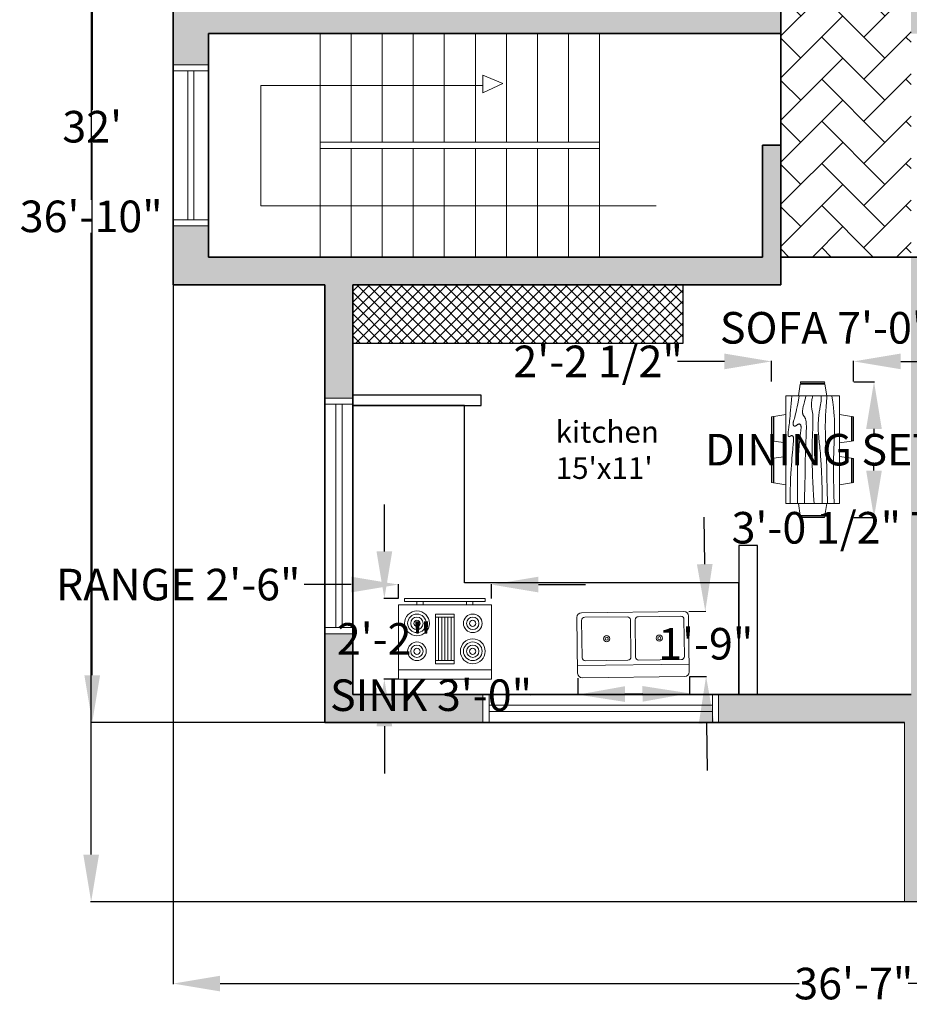
# Model space of a CAD drawing. Units: inches. Extents: x 1031 to 1706, y 87 to 654.
# Tile 1 of 4: x 1031 to 1318, y 96 to 413. Entities that reach past the tile are written whole.
import ezdxf

# ---------------------------------------------------------------- set-up
doc = ezdxf.new("R2010")
doc.units = ezdxf.units.IN
doc.header["$MEASUREMENT"] = 0
for name, color, linetype, lineweight in [('A-ANNO-DIMS', 2, 'Continuous', 18), ('A-ANNO-SYMB', 7, 'Continuous', 18), ('A-AREA-IDEN', 7, 'Continuous', 25), ('A-EQPM', 9, 'Continuous', 18), ('A-FLOR-CASE', 8, 'Continuous', 25), ('A-FLOR-CASE-PATT', 152, 'Continuous', 13), ('A-FLOR-FIXT', 114, 'Continuous', 18), ('A-FLOR-PATT', 152, 'Continuous', 13), ('A-FLOR-STRS', 7, 'Continuous', 18), ('A-FURN', 215, 'Continuous', 18), ('A-GLAZ', 4, 'Continuous', 18), ('A-WALL', 7, 'Continuous', 35), ('A-WALL-PATT', 18, 'Continuous', 13)]:
    doc.layers.add(name, color=color, linetype=linetype, lineweight=lineweight)
doc.styles.get("Standard").update_dxf_attribs({"font": 'arial.ttf'})
doc.dimstyles.get("Standard").update_dxf_attribs({"dimtxt": 10.18, "dimasz": 15.18, "dimexe": 0.18, "dimexo": 0.0625, "dimgap": 0.09, "dimtad": 0, "dimtih": 1, "dimtoh": 1, "dimdec": 0, "dimzin": 0, "dimdsep": 46, "dimlunit": 3, "dimtxsty": 'Standard', "dimcen": 0.09, "dimadec": 0, "dimazin": 0, "dimtfac": 1, "dimtdec": 0, "dimtofl": 0, "dimtmove": 0, "dimatfit": 3, "dimfxl": 1, "dimtolj": 1, "dimtzin": 0, "dimarcsym": 0})

# ---------------------------------------------------------------- blocks, each defined once
blk = doc.blocks.new('Dining Set - 36 x 72 in.')
for p, q in [((-22, 27.5), (-22.1562, 26.50042)), ((-5.8416, 26.5), (-22.1534, 26.5)), ((-22, 27.5), (-6, 27.5)), ((-5.8437, 26.49966), (-6, 27.5)), ((6, 27.5), (5.8438, 26.50042)), ((22.1584, 26.5), (5.8466, 26.5)), ((6, 27.5), (22, 27.5)), ((22.1563, 26.49966), (22, 27.5)), ((-22.2343, 26.00059), (-23.4847, 17.99762)), ((-22.2304, 26), (-5.7608, 26)), ((-4.5152, 17.99762), (-5.7655, 25.99926)), ((5.7657, 26.00059), (4.5153, 17.99762)), ((5.7696, 26), (22.2392, 26)), ((23.4848, 17.99762), (22.2345, 25.99926)), ((36, 18), (-36, 18)), ((-36, 18), (-36, -18)), ((36, -18), (36, 18)), ((-45.5, 8), (-44.5004, 8.15617)), ((-45.5, 8), (-45.5, -8)), ((-44.5, -8.15843), (-44.5, 8.15338)), ((-44.0006, 8.23428), (-35.9976, 9.48474)), ((-44, 8.23041), (-44, -8.23915)), ((44.0006, 8.23428), (35.9976, 9.48474)), ((44, 8.23041), (44, -8.23915)), ((44.5, -8.15843), (44.5, 8.15338)), ((45.5, 8), (44.5005, 8.15617)), ((45.5, 8), (45.5, -8)), ((-44.4997, -8.15631), (-45.5, -8)), ((-35.9976, -9.48476), (-43.9993, -8.2345)), ((35.9976, -9.48476), (43.9993, -8.2345)), ((44.4997, -8.15631), (45.5, -8)), ((-36, -18), (36, -18)), ((-22.2343, -26.0006), (-23.4847, -17.99762)), ((-4.5152, -17.99762), (-5.7655, -25.99928)), ((5.7657, -26.0006), (4.5153, -17.99762)), ((23.4848, -17.99762), (22.2345, -25.99928)), ((-22.2304, -26), (-5.7608, -26)), ((5.7696, -26), (22.2392, -26)), ((-22, -27.5), (-22.1562, -26.50044)), ((-5.8416, -26.5), (-22.1534, -26.5)), ((-22, -27.5), (-6, -27.5)), ((-5.8437, -26.49967), (-6, -27.5)), ((6, -27.5), (5.8438, -26.50044)), ((22.1584, -26.5), (5.8466, -26.5)), ((6, -27.5), (22, -27.5)), ((22.1563, -26.49967), (22, -27.5))]:
    blk.add_line(p, q)
for points in [[(-36, 15), (-31.1772, 14.97754), (-26.8079, 14.91406), (-22.8538, 14.81543), (-19.276, 14.6875), (-16.0362, 14.53613), (-13.0957, 14.36718), (-10.4159, 14.18652), (-7.9583, 14), (-5.6904, 13.81315), (-3.6035, 13.63021), (-1.6954, 13.45508), (0.0365, 13.29166), (1.5945, 13.14388), (2.9811, 13.01562), (4.1988, 12.9108), (5.25, 12.83333), (6.1393, 12.78613), (6.8802, 12.76823), (7.4883, 12.77767), (7.9792, 12.8125), (8.3685, 12.87077), (8.6719, 12.95052), (8.9049, 13.0498), (9.0833, 13.16666), (9.2205, 13.29899), (9.3216, 13.44401), (9.3895, 13.59879), (9.4271, 13.76041), (9.4373, 13.92594), (9.4232, 14.09245), (9.3875, 14.257), (9.3333, 14.41666), (9.2638, 14.56917), (9.1836, 14.71484), (9.0975, 14.85465), (9.0104, 14.98958), (8.9272, 15.1206), (8.8529, 15.2487), (8.7922, 15.37483), (8.75, 15.5), (8.7305, 15.62467), (8.7344, 15.74739), (8.7617, 15.86621), (8.8125, 15.97916), (8.8867, 16.08431), (8.9844, 16.17968), (9.1055, 16.26334), (9.25, 16.33333), (9.4189, 16.38802), (9.6172, 16.42708), (9.8506, 16.45052), (10.125, 16.45833), (10.4463, 16.45052), (10.8203, 16.42708), (11.2529, 16.38802), (11.75, 16.33333), (12.3184, 16.26318), (12.9694, 16.17838), (13.7151, 16.07991), (14.5677, 15.96875), (15.5395, 15.84586), (16.6426, 15.71224), (17.8893, 15.56884), (19.2917, 15.41666), (20.859, 15.25667), (22.5879, 15.08984), (24.4721, 14.91715), (26.5052, 14.73958), (28.6809, 14.5581), (30.9929, 14.3737), (33.4347, 14.18733), (36, 14)], [(-36, 10), (-28.9766, 10.14274), (-23.1725, 10.20442), (-18.4241, 10.19775), (-14.5677, 10.13541), (-11.4399, 10.03011), (-8.877, 9.89453), (-6.7154, 9.74137), (-4.7917, 9.58333), (-2.9698, 9.43082), (-1.2246, 9.28515), (0.4415, 9.14534), (2.026, 9.01041), (3.5266, 8.87939), (4.9408, 8.7513), (6.266, 8.62516), (7.5, 8.5), (8.6411, 8.37549), (9.6914, 8.2539), (10.6538, 8.13818), (11.5312, 8.03125), (12.3267, 7.93603), (13.043, 7.85547), (13.6831, 7.79248), (14.25, 7.75), (14.7471, 7.7303), (15.1797, 7.73307), (15.5537, 7.75732), (15.875, 7.80208), (16.1494, 7.86637), (16.3828, 7.94922), (16.5811, 8.04964), (16.75, 8.16666), (16.8944, 8.29915), (17.0143, 8.44531), (17.1089, 8.60319), (17.1771, 8.77083), (17.218, 8.94629), (17.2305, 9.1276), (17.2137, 9.31282), (17.1667, 9.5), (17.0895, 9.6875), (16.987, 9.875), (16.8649, 10.0625), (16.7292, 10.25), (16.5856, 10.4375), (16.4401, 10.625), (16.2985, 10.8125), (16.1667, 11), (16.05, 11.18733), (15.9518, 11.3737), (15.8752, 11.5581), (15.8229, 11.73958), (15.798, 11.91715), (15.8034, 12.08984), (15.842, 12.25667), (15.9167, 12.41666), (16.0295, 12.56836), (16.1784, 12.70833), (16.3605, 12.83268), (16.5729, 12.9375), (16.8127, 13.01888), (17.0768, 13.07291), (17.3625, 13.0957), (17.6667, 13.08333), (17.9894, 13.03312), (18.3418, 12.94726), (18.7382, 12.82918), (19.1927, 12.68229), (19.7195, 12.51001), (20.3327, 12.31575), (21.0465, 12.10294), (21.875, 11.875), (22.8357, 11.63354), (23.959, 11.37304), (25.2786, 11.08618), (26.8282, 10.76562), (28.6414, 10.40405), (30.752, 9.99414), (33.1936, 9.52856), (36, 9)], [(-36, 5.5), (-30.7157, 5.3348), (-26.069, 5.20963), (-21.9946, 5.11767), (-18.4271, 5.05208), (-15.3009, 5.00602), (-12.5508, 4.97265), (-10.1112, 4.94515), (-7.9167, 4.91666), (-5.909, 4.88167), (-4.0586, 4.83984), (-2.3429, 4.79215), (-0.7396, 4.73958), (0.7739, 4.6831), (2.22, 4.6237), (3.6213, 4.56233), (5, 4.5), (6.373, 4.43782), (7.7344, 4.3776), (9.0723, 4.32129), (10.375, 4.27083), (11.6309, 4.22819), (12.8281, 4.19531), (13.9551, 4.17415), (15, 4.16666), (15.954, 4.17448), (16.819, 4.19791), (17.6001, 4.23698), (18.3021, 4.29166), (18.9299, 4.36198), (19.4883, 4.44791), (19.9823, 4.54948), (20.4167, 4.66666), (20.7969, 4.79899), (21.1302, 4.94401), (21.4245, 5.09879), (21.6875, 5.26041), (21.9271, 5.42594), (22.1511, 5.59245), (22.3672, 5.757), (22.5834, 5.91666), (22.8065, 6.06868), (23.0404, 6.21093), (23.2879, 6.34147), (23.5521, 6.45833), (23.8358, 6.55957), (24.142, 6.64323), (24.4735, 6.70735), (24.8334, 6.75), (25.2235, 6.76969), (25.642, 6.76692), (26.0858, 6.74267), (26.5521, 6.69791), (27.0379, 6.63362), (27.5404, 6.55078), (28.0565, 6.45036), (28.5834, 6.33333), (29.1242, 6.19987), (29.7071, 6.04687), (30.3661, 5.87044), (31.1354, 5.66666), (32.0493, 5.43164), (33.142, 5.16146), (34.4475, 4.85221), (36, 4.5)], [(-36, -1), (-30.7915, -0.6591), (-26.0195, -0.38216), (-21.6519, -0.16284), (-17.6563, 0.00521), (-14.0005, 0.12833), (-10.6523, 0.21289), (-7.5796, 0.26522), (-4.75, 0.29166), (-2.134, 0.29793), (0.2878, 0.28711), (2.5317, 0.26163), (4.6146, 0.22396), (6.5529, 0.17651), (8.3633, 0.12174), (10.0623, 0.06209), (11.6667, 0), (13.1899, -0.06201), (14.6341, -0.1211), (15.9982, -0.17432), (17.2813, -0.21875), (18.4823, -0.25147), (19.6003, -0.26953), (20.6343, -0.27002), (21.5834, -0.25), (22.4481, -0.20768), (23.2357, -0.14584), (23.9549, -0.06836), (24.6146, 0.02083), (25.2235, 0.11784), (25.7904, 0.21875), (26.3241, 0.31966), (26.8334, 0.41666), (27.3265, 0.50618), (27.8099, 0.58593), (28.2894, 0.65397), (28.7709, 0.70833), (29.2601, 0.74707), (29.763, 0.76823), (30.2855, 0.76985), (30.8334, 0.75), (31.4088, 0.70784), (31.9994, 0.64713), (32.589, 0.57275), (33.1615, 0.48958), (33.7008, 0.4025), (34.1908, 0.3164), (34.6153, 0.23616), (34.9584, 0.16666), (35.2099, 0.11165), (35.3848, 0.07031), (35.504, 0.04069), (35.5886, 0.02083), (35.6594, 0.00879), (35.7377, 0.0026), (35.8442, 0.00032), (36, 0)], [(-36, -6.5), (-27.1843, -6.31267), (-20.084, -6.1263), (-14.469, -5.9419), (-10.1094, -5.76042), (-6.7752, -5.58285), (-4.2363, -5.41016), (-2.2629, -5.24333), (-0.625, -5.08334), (0.8708, -4.93099), (2.2715, -4.78646), (3.5872, -4.64974), (4.8281, -4.52084), (6.0046, -4.39974), (7.127, -4.28646), (8.2053, -4.18099), (9.25, -4.08334), (10.2705, -3.99382), (11.2734, -3.91407), (12.2647, -3.84603), (13.25, -3.79167), (14.2354, -3.75293), (15.2266, -3.73177), (16.2295, -3.73015), (17.25, -3.75), (18.2912, -3.79248), (19.3451, -3.85547), (20.4009, -3.93604), (21.4479, -4.03125), (22.4754, -4.13819), (23.4727, -4.25391), (24.4289, -4.37549), (25.3334, -4.5), (26.1785, -4.62492), (26.9694, -4.74935), (27.7145, -4.87281), (28.4219, -4.99479), (29.1, -5.11483), (29.7572, -5.23242), (30.4016, -5.34709), (31.0417, -5.45834), (31.6837, -5.56437), (32.3262, -5.65821), (32.9658, -5.73153), (33.599, -5.77604), (34.2224, -5.78345), (34.8327, -5.74545), (35.4264, -5.65373), (36, -5.5)], [(-36, -10), (-26.4022, -9.81299), (-18.4675, -9.62891), (-11.9839, -9.45069), (-6.7396, -9.28125), (-2.5226, -9.12354), (0.8789, -8.98047), (3.6769, -8.85498), (6.0833, -8.75), (8.2767, -8.66765), (10.3021, -8.60677), (12.1712, -8.56543), (13.8958, -8.54167), (15.4876, -8.53353), (16.9583, -8.53907), (18.3197, -8.55632), (19.5834, -8.58334), (20.7616, -8.61841), (21.8685, -8.66081), (22.9188, -8.71004), (23.9271, -8.76563), (24.9081, -8.82707), (25.8763, -8.89388), (26.8465, -8.96558), (27.8334, -9.04167), (28.8474, -9.12118), (29.8828, -9.20117), (30.93, -9.27824), (31.9792, -9.34896), (33.0205, -9.40991), (34.0443, -9.45768), (35.0407, -9.48885), (36, -9.5)], [(-36, -14.5), (-30.0881, -14.33513), (-25.0332, -14.21224), (-20.7312, -14.12647), (-17.0781, -14.07292), (-13.97, -14.04671), (-11.3027, -14.04297), (-8.9724, -14.05681), (-6.875, -14.08334), (-4.9224, -14.11833), (-3.0905, -14.16016), (-1.3709, -14.20785), (0.2448, -14.26042), (1.7647, -14.3169), (3.1973, -14.3763), (4.5507, -14.43767), (5.8333, -14.5), (7.0554, -14.5621), (8.235, -14.62175), (9.3922, -14.67652), (10.5469, -14.72396), (11.7192, -14.76164), (12.929, -14.78711), (14.1965, -14.79794), (15.5417, -14.79167), (16.9933, -14.76424), (18.6152, -14.70508), (20.4804, -14.60197), (22.6615, -14.44271), (25.2312, -14.21509), (28.2624, -13.9069), (31.8277, -13.50594), (36, -13)]]:
    blk.add_lwpolyline(points)
blk = doc.blocks.new('Range-Oven - 30 in top')
for p, q in [((0, -3), (30, -3)), ((12, -6), (18, -6)), ((13, -20), (13, -6)), ((14, -6), (14, -20)), ((15, -20), (15, -6)), ((16, -6), (16, -20)), ((17, -20), (17, -6)), ((18, -20), (12, -20)), ((6, -24), (6, -25)), ((8, -25), (8, -24)), ((22, -25), (22, -24)), ((24, -24), (24, -25))]:
    blk.add_line(p, q)
for points in [[(0, -24), (0, 0), (30, 0), (30, -24)], [(12, -21), (12, -5), (18, -5), (18, -21)], [(2, -26), (2, -25), (28, -25), (28, -26)]]:
    blk.add_lwpolyline(points, close=True)
for centre, radius in [((6, -9), 4), ((6, -9), 3), ((24, -9), 3), ((6, -9), 2), ((6, -9), 1), ((24, -9), 2), ((24, -9), 1), ((6, -18), 3), ((24, -18), 4), ((24, -18), 3), ((6, -18), 2), ((6, -18), 1), ((24, -18), 2), ((24, -18), 1)]:
    blk.add_circle(centre, radius)
blk = doc.blocks.new('Sink-double - 36 in top')
for p, q in [((-18, -4), (18, -4)), ((-0.75, -18.5), (-0.75, -6.5)), ((0.75, -6.5), (0.75, -18.5))]:
    blk.add_line(p, q)
for points in [[(-16.5, 0), (16.5, 0)], [(-18, -19.5), (-18, -1.5)], [(18, -1.5), (18, -19.5)], [(-15.5, -5.5), (-1.75, -5.5)], [(1.75, -5.5), (15.5, -5.5)], [(-16.5, -18.5), (-16.5, -6.5)], [(16.5, -6.5), (16.5, -18.5)], [(16.5, -21), (-16.5, -21)], [(-1.75, -19.5), (-15.5, -19.5)], [(15.5, -19.5), (1.75, -19.5)]]:
    blk.add_lwpolyline(points)
for centre, radius in [((-8.5, -12.5), 1), ((-8.5, -12.5), 0.5), ((8.5, -12.5), 1), ((8.5, -12.5), 0.5)]:
    blk.add_circle(centre, radius)
for centre, radius, start, end in [((-16.5, -1.5), 1.5, 90, 180), ((16.5, -1.5), 1.5, 0, 90), ((-15.5, -6.5), 1, 90, 180), ((-1.75, -6.5), 1, 0, 90), ((1.75, -6.5), 1, 90, 180), ((15.5, -6.5), 1, 0, 90), ((-15.5, -18.5), 1, 180, 270), ((-1.75, -18.5), 1, 270, 0), ((1.75, -18.5), 1, 180, 270), ((15.5, -18.5), 1, 270, 0), ((-16.5, -19.5), 1.5, 180, 270), ((16.5, -19.5), 1.5, 270, 0)]:
    blk.add_arc(centre, radius, start, end)
blk = doc.blocks.new('*D13')
at = {"layer": 'A-ANNO-DIMS', "color": 0, "lineweight": -2, "transparency": 16777216}
for p, q in [((1129.54, 570.4), (1054.37, 570.4)), ((1054.55, 555.22), (1054.55, 383.69)), ((1054.55, 201.58), (1054.55, 373.11)), ((1129.54, 186.4), (1054.37, 186.4))]:
    blk.add_line(p, q, dxfattribs=at)
at = {"layer": 'A-ANNO-DIMS', "color": 0, "transparency": 16777216}
for points in [[(1052.02, 555.22), (1057.08, 555.22), (1054.55, 570.4)], [(1052.02, 201.58), (1057.08, 201.58), (1054.55, 186.4)]]:
    blk.add_solid(points, dxfattribs=at)
at = {"layer": 'Defpoints', "color": 0, "transparency": 16777216}
for p in [(1129.6, 570.4), (1054.55, 186.4), (1129.6, 186.4)]:
    blk.add_point(p, dxfattribs=at)
at = {"layer": 'A-ANNO-DIMS', "color": 0, "transparency": 16777216, "insert": (1054.55, 378.4), "char_height": 10.18, "attachment_point": 5}
blk.add_mtext("\\A1;32'", dxfattribs=at)
blk = doc.blocks.new('WIN-72IN')
for p, q in [((0, 0), (0, 9)), ((2, 0), (2, 9)), ((74, 0), (74, 9)), ((76, 0), (76, 9)), ((2, 5.5), (74, 5.5)), ((2, 3.5), (74, 3.5))]:
    blk.add_line(p, q)
blk = doc.blocks.new('*D28')
at = {"layer": 'A-ANNO-DIMS', "color": 0, "lineweight": -2, "transparency": 16777216}
for p, q in [((1374.5, 313.58), (1359.32, 313.58)), ((1374.5, 301.04), (1374.5, 313.76)), ((1443.32, 313.58), (1389.68, 313.58)), ((1458.5, 301.04), (1458.5, 313.76))]:
    blk.add_line(p, q, dxfattribs=at)
at = {"layer": 'A-ANNO-DIMS', "color": 0, "transparency": 16777216}
for points in [[(1389.68, 316.11), (1389.68, 311.05), (1374.5, 313.58)], [(1443.32, 316.11), (1443.32, 311.05), (1458.5, 313.58)]]:
    blk.add_solid(points, dxfattribs=at)
at = {"layer": 'Defpoints', "color": 0, "transparency": 16777216}
for p in [(1374.5, 313.58), (1374.5, 300.98), (1458.5, 300.98)]:
    blk.add_point(p, dxfattribs=at)
at = {"layer": 'A-ANNO-DIMS', "color": 0, "transparency": 16777216, "insert": (1306.9, 313.58), "char_height": 10.18, "attachment_point": 5}
blk.add_mtext('\\A1;SOFA 7\'-0" TYP.', dxfattribs=at)
blk = doc.blocks.new('*D29')
at = {"layer": 'A-ANNO-DIMS', "color": 0, "lineweight": -2, "transparency": 16777216}
for p, q in [((1374.44, 300.98), (1361.72, 300.98)), ((1361.9, 285.8), (1361.9, 279.49)), ((1374.44, 264.31), (1361.72, 264.31)), ((1361.9, 264.31), (1361.9, 249.13)), ((1361.9, 249.13), (1346.72, 249.13))]:
    blk.add_line(p, q, dxfattribs=at)
at = {"layer": 'A-ANNO-DIMS', "color": 0, "transparency": 16777216}
for points in [[(1359.37, 285.8), (1364.43, 285.8), (1361.9, 300.98)], [(1359.37, 279.49), (1364.43, 279.49), (1361.9, 264.31)]]:
    blk.add_solid(points, dxfattribs=at)
at = {"layer": 'Defpoints', "color": 0, "transparency": 16777216}
for p in [(1374.5, 300.98), (1361.9, 264.31), (1374.5, 264.31)]:
    blk.add_point(p, dxfattribs=at)
at = {"layer": 'A-ANNO-DIMS', "color": 0, "transparency": 16777216, "insert": (1303.75, 249.13), "char_height": 10.18, "attachment_point": 5}
blk.add_mtext('\\A1;3\'-0 1/2" TYP.', dxfattribs=at)
blk = doc.blocks.new('*D30')
at = {"layer": 'A-ANNO-DIMS', "color": 0, "lineweight": -2, "transparency": 16777216}
for p, q in [((1300.12, 296.19), (1306.8, 296.19)), ((1306.62, 281.01), (1306.62, 279.65)), ((1306.62, 267.58), (1306.62, 268.93)), ((1300.12, 252.4), (1306.8, 252.4))]:
    blk.add_line(p, q, dxfattribs=at)
at = {"layer": 'A-ANNO-DIMS', "color": 0, "transparency": 16777216}
for points in [[(1304.09, 281.01), (1309.15, 281.01), (1306.62, 296.19)], [(1304.09, 267.58), (1309.15, 267.58), (1306.62, 252.4)]]:
    blk.add_solid(points, dxfattribs=at)
at = {"layer": 'Defpoints', "color": 0, "transparency": 16777216}
for p in [(1300.06, 296.19), (1306.62, 296.19), (1300.06, 252.4)]:
    blk.add_point(p, dxfattribs=at)
at = {"layer": 'A-ANNO-DIMS', "color": 0, "transparency": 16777216, "insert": (1306.62, 274.29), "char_height": 10.18, "attachment_point": 5}
blk.add_mtext('\\A1;DINING SET 3\'-8"', dxfattribs=at)
blk = doc.blocks.new('*D31')
at = {"layer": 'A-ANNO-DIMS', "color": 0, "lineweight": -2, "transparency": 16777216}
for p, q in [((1258.41, 302.75), (1243.23, 302.75)), ((1273.59, 296.25), (1273.59, 302.93)), ((1300.06, 296.25), (1300.06, 302.93)), ((1315.24, 302.75), (1330.42, 302.75))]:
    blk.add_line(p, q, dxfattribs=at)
at = {"layer": 'A-ANNO-DIMS', "color": 0, "transparency": 16777216}
for points in [[(1258.41, 305.28), (1258.41, 300.22), (1273.59, 302.75)], [(1315.24, 305.28), (1315.24, 300.22), (1300.06, 302.75)]]:
    blk.add_solid(points, dxfattribs=at)
at = {"layer": 'Defpoints', "color": 0, "transparency": 16777216}
for p in [(1273.59, 302.75), (1273.59, 296.19), (1300.06, 296.19)]:
    blk.add_point(p, dxfattribs=at)
at = {"layer": 'A-ANNO-DIMS', "color": 0, "transparency": 16777216, "insert": (1217.66, 302.75), "char_height": 10.18, "attachment_point": 5}
blk.add_mtext('\\A1;2\'-2 1/2"', dxfattribs=at)
blk = doc.blocks.new('*D34')
at = {"layer": 'A-ANNO-DIMS', "color": 0, "lineweight": -2, "transparency": 16777216}
for p, q in [((1138.07, 230.82), (1122.89, 230.82)), ((1153.25, 226.38), (1153.25, 231)), ((1183.25, 226.38), (1183.25, 231)), ((1198.43, 230.82), (1213.61, 230.82))]:
    blk.add_line(p, q, dxfattribs=at)
at = {"layer": 'A-ANNO-DIMS', "color": 0, "transparency": 16777216}
for points in [[(1138.07, 233.35), (1138.07, 228.29), (1153.25, 230.82)], [(1198.43, 233.35), (1198.43, 228.29), (1183.25, 230.82)]]:
    blk.add_solid(points, dxfattribs=at)
at = {"layer": 'Defpoints', "color": 0, "transparency": 16777216}
for p in [(1153.25, 230.82), (1153.25, 226.32), (1183.25, 226.32)]:
    blk.add_point(p, dxfattribs=at)
at = {"layer": 'A-ANNO-DIMS', "color": 0, "transparency": 16777216, "insert": (1082.27, 230.82), "char_height": 10.18, "attachment_point": 5}
blk.add_mtext('\\A1;RANGE 2\'-6"', dxfattribs=at)
blk = doc.blocks.new('*D35')
at = {"layer": 'A-ANNO-DIMS', "color": 0, "lineweight": -2, "transparency": 16777216}
for p, q in [((1148.75, 241.5), (1148.75, 256.68)), ((1153.18, 226.32), (1148.57, 226.32)), ((1153.18, 200.32), (1148.57, 200.32)), ((1148.75, 185.14), (1148.75, 169.96))]:
    blk.add_line(p, q, dxfattribs=at)
at = {"layer": 'A-ANNO-DIMS', "color": 0, "transparency": 16777216}
for points in [[(1146.22, 241.5), (1151.28, 241.5), (1148.75, 226.32)], [(1146.22, 185.14), (1151.28, 185.14), (1148.75, 200.32)]]:
    blk.add_solid(points, dxfattribs=at)
at = {"layer": 'Defpoints', "color": 0, "transparency": 16777216}
for p in [(1153.25, 226.32), (1148.75, 200.32), (1153.25, 200.32)]:
    blk.add_point(p, dxfattribs=at)
at = {"layer": 'A-ANNO-DIMS', "color": 0, "transparency": 16777216, "insert": (1148.75, 213.32), "char_height": 10.18, "attachment_point": 5}
blk.add_mtext('\\A1;2\'-2"', dxfattribs=at)
blk = doc.blocks.new('*D36')
at = {"layer": 'A-ANNO-DIMS', "color": 0, "lineweight": -2, "transparency": 16777216}
for p, q in [((1211.08, 200.68), (1211.15, 195.16)), ((1247.08, 201.11), (1247.15, 195.59)), ((1211.15, 195.34), (1195.97, 195.16)), ((1231.97, 195.59), (1226.33, 195.52))]:
    blk.add_line(p, q, dxfattribs=at)
at = {"layer": 'A-ANNO-DIMS', "color": 0, "transparency": 16777216}
for points in [[(1226.3, 198.05), (1226.36, 192.99), (1211.15, 195.34)], [(1231.94, 198.12), (1232, 193.06), (1247.14, 195.77)]]:
    blk.add_solid(points, dxfattribs=at)
at = {"layer": 'Defpoints', "color": 0, "transparency": 16777216}
for p in [(1211.08, 200.74), (1247.08, 201.17), (1211.15, 195.34)]:
    blk.add_point(p, dxfattribs=at)
at = {"layer": 'A-ANNO-DIMS', "color": 0, "transparency": 16777216, "insert": (1163.8, 195.16), "char_height": 10.18, "attachment_point": 5}
blk.add_mtext('\\A1;SINK 3\'-0"', dxfattribs=at)
blk = doc.blocks.new('*D37')
at = {"layer": 'A-ANNO-DIMS', "color": 0, "lineweight": -2, "transparency": 16777216}
for p, q in [((1252.05, 237.41), (1251.87, 252.59)), ((1246.89, 222.17), (1252.41, 222.23)), ((1247.14, 201.17), (1252.66, 201.23)), ((1252.66, 186.05), (1252.84, 170.87))]:
    blk.add_line(p, q, dxfattribs=at)
at = {"layer": 'A-ANNO-DIMS', "color": 0, "transparency": 16777216}
for points in [[(1254.58, 237.44), (1249.52, 237.38), (1252.23, 222.23)], [(1255.19, 186.08), (1250.13, 186.02), (1252.48, 201.23)]]:
    blk.add_solid(points, dxfattribs=at)
at = {"layer": 'Defpoints', "color": 0, "transparency": 16777216}
for p in [(1246.83, 222.17), (1247.08, 201.17), (1252.48, 201.23)]:
    blk.add_point(p, dxfattribs=at)
at = {"layer": 'A-ANNO-DIMS', "color": 0, "transparency": 16777216, "insert": (1252.36, 211.73), "char_height": 10.18, "attachment_point": 5}
blk.add_mtext('\\A1;1\'-9"', dxfattribs=at)
blk = doc.blocks.new('*D40')
at = {"layer": 'A-ANNO-DIMS', "color": 0, "lineweight": -2, "transparency": 16777216}
for p, q in [((1080.61, 327.33), (1080.61, 102.02)), ((1519.6, 186.33), (1519.6, 102.02)), ((1095.79, 102.2), (1282.53, 102.2)), ((1504.42, 102.2), (1317.68, 102.2))]:
    blk.add_line(p, q, dxfattribs=at)
at = {"layer": 'A-ANNO-DIMS', "color": 0, "transparency": 16777216}
for points in [[(1095.79, 104.73), (1095.79, 99.67), (1080.61, 102.2)], [(1504.42, 104.73), (1504.42, 99.67), (1519.6, 102.2)]]:
    blk.add_solid(points, dxfattribs=at)
at = {"layer": 'Defpoints', "color": 0, "transparency": 16777216}
for p in [(1080.61, 327.4), (1519.6, 186.4), (1519.6, 102.2)]:
    blk.add_point(p, dxfattribs=at)
at = {"layer": 'A-ANNO-DIMS', "color": 0, "transparency": 16777216, "insert": (1300.1, 102.2), "char_height": 10.18, "attachment_point": 5}
blk.add_mtext('\\A1;36\'-7"', dxfattribs=at)
blk = doc.blocks.new('*D41')
at = {"layer": 'A-ANNO-DIMS', "color": 0, "lineweight": -2, "transparency": 16777216}
for p, q in [((1129.54, 570.4), (1054.03, 570.4)), ((1054.21, 555.22), (1054.21, 354.79)), ((1054.21, 143.78), (1054.21, 344.21)), ((1324.54, 128.6), (1054.03, 128.6))]:
    blk.add_line(p, q, dxfattribs=at)
at = {"layer": 'A-ANNO-DIMS', "color": 0, "transparency": 16777216}
for points in [[(1051.68, 555.22), (1056.74, 555.22), (1054.21, 570.4)], [(1051.68, 143.78), (1056.74, 143.78), (1054.21, 128.6)]]:
    blk.add_solid(points, dxfattribs=at)
at = {"layer": 'Defpoints', "color": 0, "transparency": 16777216}
for p in [(1054.21, 570.4), (1129.6, 570.4), (1324.6, 128.6)]:
    blk.add_point(p, dxfattribs=at)
at = {"layer": 'A-ANNO-DIMS', "color": 0, "transparency": 16777216, "insert": (1054.21, 349.5), "char_height": 10.18, "attachment_point": 5}
blk.add_mtext('\\A1;36\'-10"', dxfattribs=at)

msp = doc.modelspace()

# ---------------------------------------------------------------- hatches: boundary and pattern name
at = {"layer": 'A-FLOR-CASE-PATT'}
h = msp.add_hatch(dxfattribs=at)
h.set_pattern_fill('ANSI37', color=256, scale=20)
h.paths.add_polyline_path([(1244.94, 327.4), (1138.6, 327.4), (1138.6, 308.56), (1244.94, 308.56)])
at = {"layer": 'A-FLOR-PATT'}
h = msp.add_hatch(dxfattribs=at)
h.set_pattern_fill('AR-HBONE', color=256, scale=2.4)
h.paths.add_polyline_path([(1372.6, 507.4), (1330.6, 507.4), (1330.6, 471.4), (1276.6, 471.4), (1276.6, 408.4), (1276.6, 336.4), (1318.6, 336.4), (1318.6, 417.4), (1372.6, 417.4)])
at = {"layer": 'A-WALL-PATT'}
h = msp.add_hatch(color=256, dxfattribs=at)
h.dxf.hatch_style = 1
h.paths.add_polyline_path([(1324.6, 336.4), (1318.6, 336.4), (1318.6, 327.4), (1318.6, 195.4), (1256.53, 195.4), (1256.53, 186.4), (1316.43, 186.4), (1316.43, 128.6), (1324.6, 128.6), (1324.6, 142.78), (1421.89, 142.78), (1421.89, 143.49), (1324.6, 143.49), (1324.6, 157.67), (1324.6, 171.8), (1421.89, 171.8), (1421.89, 172.21), (1324.6, 172.21), (1324.6, 186.4)])
h.paths.add_polyline_path([(1378.07, 258.4), (1358.04, 258.4), (1358.04, 249.4), (1378.07, 249.4)], flags=17)
h.paths.add_polyline_path([(1519.6, 299.69), (1510.6, 299.69), (1510.6, 258.4), (1454.07, 258.4), (1454.07, 249.4), (1519.6, 249.4)])
h.paths.add_polyline_path([(1519.6, 456.87), (1510.6, 456.87), (1510.6, 417.4), (1372.6, 417.4), (1318.6, 417.4), (1318.6, 408.4), (1510.6, 408.4), (1510.6, 375.69), (1519.6, 375.69)])
h.paths.add_polyline_path([(1276.6, 372.4), (1270.65, 372.4), (1270.65, 336.4), (1138.6, 336.4), (1092.08, 336.4), (1092.08, 346.4), (1080.61, 346.4), (1080.61, 327.4), (1129.6, 327.4), (1129.6, 290.93), (1138.6, 290.93), (1138.6, 291.84), (1138.6, 327.4), (1244.94, 327.4), (1276.6, 327.4)])
h.paths.add_polyline_path([(1276.6, 417.4), (1138.6, 417.4), (1138.6, 438.03), (1129.6, 438.03), (1129.6, 417.4), (1080.61, 417.4), (1080.61, 398.4), (1092.08, 398.4), (1092.08, 408.4), (1138.6, 408.4), (1276.6, 408.4)])
h.paths.add_polyline_path([(1180.53, 195.4), (1138.6, 195.4), (1138.6, 214.93), (1129.6, 214.93), (1129.6, 186.4), (1180.53, 186.4)])
h.paths.add_polyline_path([(1519.6, 570.4), (1489.02, 570.4), (1489.02, 561.4), (1510.6, 561.4), (1510.6, 532.87), (1519.6, 532.87)])
h.paths.add_polyline_path([(1413.02, 570.4), (1365.47, 570.4), (1365.47, 561.4), (1372.6, 561.4), (1372.6, 507.4), (1372.6, 417.4), (1378.6, 417.4), (1378.6, 561.4), (1413.02, 561.4)])
h.paths.add_polyline_path([(1289.42, 570.4), (1242.6, 570.4), (1242.6, 561.4), (1270.6, 561.4), (1270.6, 471.4), (1291.02, 471.4), (1291.02, 477.4), (1276.6, 477.4), (1276.6, 561.4), (1289.42, 561.4)])
h.paths.add_polyline_path([(1337.47, 570.4), (1317.42, 570.4), (1317.42, 561.4), (1324.6, 561.4), (1324.6, 471.4), (1330.6, 471.4), (1330.6, 507.4), (1338.54, 507.4), (1338.54, 513.4), (1330.6, 513.4), (1330.6, 561.4), (1337.47, 561.4)])
h.paths.add_polyline_path([(1138.6, 561.4), (1166.6, 561.4), (1166.6, 570.4), (1129.6, 570.4), (1129.6, 514.03), (1138.6, 514.03)])

# ---------------------------------------------------------------- linework, layer by layer
at = {"layer": 'A-ANNO-SYMB'}
for p, q in [((1180.54, 391.72), (1180.54, 395.02)), ((1180.54, 395.02), (1180.54, 389.29)), ((1186.96, 392.29), (1180.54, 395.02)), ((1108.95, 352.9), (1108.95, 391.72)), ((1108.95, 391.72), (1180.54, 391.72)), ((1180.54, 389.29), (1186.96, 392.29)), ((1236.35, 352.9), (1108.95, 352.9))]:
    msp.add_line(p, q, dxfattribs=at)
at = {"layer": 'A-FLOR-CASE'}
for p, q in [((1174.6, 288.53), (1138.6, 288.53)), ((1174.6, 231.4), (1174.6, 288.53)), ((1263.09, 231.4), (1174.6, 231.4)), ((1263.09, 195.4), (1263.09, 231.4))]:
    msp.add_line(p, q, dxfattribs=at)
for points in [[(1138.6, 327.4), (1244.94, 327.4), (1244.94, 308.56), (1138.6, 308.56)], [(1138.6, 288.53), (1179.95, 288.53), (1179.95, 291.84), (1138.6, 291.84)], [(1263.09, 195.4), (1269.11, 195.4), (1269.11, 243.41), (1263.09, 243.41)]]:
    msp.add_lwpolyline(points, close=True, dxfattribs=at)
at = {"layer": 'A-FLOR-STRS'}
for p, q in [((1128.08, 408.4), (1128.08, 336.4)), ((1138.08, 408.4), (1138.08, 373.4)), ((1148.08, 408.4), (1148.08, 373.4)), ((1158.08, 408.4), (1158.08, 373.4)), ((1168.08, 408.4), (1168.08, 373.4)), ((1178.08, 408.4), (1178.08, 373.4)), ((1188.08, 408.4), (1188.08, 373.4)), ((1198.08, 408.4), (1198.08, 373.4)), ((1208.08, 408.4), (1208.08, 373.4)), ((1218.08, 408.4), (1218.08, 336.4)), ((1128.08, 373.4), (1218.08, 373.4)), ((1128.08, 371.4), (1218.08, 371.4)), ((1138.08, 371.4), (1138.08, 336.4)), ((1148.08, 371.4), (1148.08, 336.4)), ((1158.08, 371.4), (1158.08, 336.4)), ((1168.08, 371.4), (1168.08, 336.4)), ((1178.08, 371.4), (1178.08, 336.4)), ((1188.08, 371.4), (1188.08, 336.4)), ((1198.08, 371.4), (1198.08, 336.4)), ((1208.08, 371.4), (1208.08, 336.4)), ((1316.43, 186.4), (1316.43, 128.6)), ((1316.43, 128.6), (1324.6, 128.6))]:
    msp.add_line(p, q, dxfattribs=at)
at = {"layer": 'A-GLAZ'}
for p, q in [((1092.08, 398.4), (1080.61, 398.4)), ((1092.08, 396.4), (1080.61, 396.4)), ((1085.34, 348.4), (1085.34, 396.4)), ((1087.34, 348.4), (1087.34, 396.4)), ((1092.08, 376.49), (1092.08, 376.49)), ((1092.08, 348.4), (1080.61, 348.4)), ((1092.08, 346.4), (1080.61, 346.4))]:
    msp.add_line(p, q, dxfattribs=at)
at = {"layer": 'A-WALL'}
for p, q in [((1276.6, 408.4), (1276.6, 471.4)), ((1080.61, 417.4), (1080.61, 327.4)), ((1138.6, 408.4), (1092.08, 408.4)), ((1092.08, 408.4), (1092.08, 336.4)), ((1138.6, 408.4), (1276.6, 408.4)), ((1276.6, 408.4), (1276.6, 327.4)), ((1270.65, 372.4), (1270.65, 336.4)), ((1270.65, 372.4), (1276.6, 372.4)), ((1092.08, 336.4), (1138.6, 336.4)), ((1270.65, 336.4), (1138.6, 336.4)), ((1324.6, 336.4), (1276.6, 336.4)), ((1080.61, 327.4), (1129.6, 327.4)), ((1129.6, 186.4), (1129.6, 327.4)), ((1138.6, 195.4), (1138.6, 327.4)), ((1276.6, 327.4), (1138.6, 327.4)), ((1318.6, 195.4), (1138.6, 195.4)), ((1316.43, 186.4), (1129.6, 186.4))]:
    msp.add_line(p, q, dxfattribs=at)

# ---------------------------------------------------------------- block references
at = {"layer": 'A-EQPM', "rotation": 180}
msp.add_blockref('Range-Oven - 30 in top', (1183.25, 200.32), dxfattribs=at)
at = {"layer": 'A-FLOR-FIXT', "rotation": 180.6822162996}
msp.add_blockref('Sink-double - 36 in top', (1229.08, 200.95), dxfattribs=at)
at = {"layer": 'A-FURN', "xscale": 0.4811908207601908, "yscale": 0.4811908207601908, "zscale": 0.4811908207601908, "rotation": 90}
msp.add_blockref('Dining Set - 36 x 72 in.', (1286.82, 274.29), dxfattribs=at)
at = {"layer": 'A-GLAZ'}
for p, rotation in [((1138.6, 214.93), 90.00000000000021), ((1256.53, 195.4), 180)]:
    msp.add_blockref('WIN-72IN', p, dxfattribs=dict(at, rotation=rotation))

# ---------------------------------------------------------------- texts
at = {"layer": 'A-AREA-IDEN', "insert": (1203.98, 283.54), "char_height": 7, "attachment_point": 1}
msp.add_mtext_dynamic_manual_height_columns("kitchen\\P15'x11'", width=113.8004, gutter_width=1, heights=[0], dxfattribs=at)

# ---------------------------------------------------------------- dimensions: what is measured, and where the dimension line sits
at = {"layer": 'A-ANNO-DIMS'}
for base, p1, p2, angle, override, picture, middle in [((1054.21, 570.4), (1324.6, 128.6), (1129.6, 570.4), 90, {"dimdec": 1, "dimlfac": 1, "dimrnd": 0, "dimzin": 1, "dimdsep": 46, "dimlunit": 4, "dimfrac": 2}, '*D41', (1054.21, 349.5)), ((1054.55, 186.4), (1129.6, 570.4), (1129.6, 186.4), 90, {"dimclrd": 0, "dimclre": 0, "dimclrt": 0}, '*D13', (1054.55, 378.4)), ((1273.59, 302.75), (1300.06, 296.19), (1273.59, 296.19), 180, {"dimdec": 1, "dimlfac": 1, "dimrnd": 0, "dimzin": 1, "dimdsep": 46, "dimlunit": 4, "dimfrac": 2}, '*D31', (1217.66, 302.75)), ((1148.75, 200.32), (1153.25, 226.32), (1153.25, 200.32), 270, {"dimdec": 1, "dimlfac": 1, "dimrnd": 0, "dimzin": 1, "dimdsep": 46, "dimlunit": 4, "dimfrac": 2}, '*D35', (1148.75, 213.32)), ((1252.48, 201.23), (1246.83, 222.17), (1247.08, 201.17), 270.6822, {"dimdec": 1, "dimlfac": 1, "dimrnd": 0, "dimzin": 1, "dimdsep": 46, "dimlunit": 4, "dimfrac": 2}, '*D37', (1252.36, 211.73))]:
    dim = msp.add_linear_dim(base=base, p1=p1, p2=p2, angle=angle, dimstyle='Standard', override=override, dxfattribs=at)
    dim.commit()
    dim.dimension.update_dxf_attribs({"geometry": picture, "text_midpoint": middle})
for base, p1, p2, angle, text, picture, middle in [((1374.5, 313.58), (1458.5, 300.98), (1374.5, 300.98), 180, 'SOFA <> TYP.', '*D28', (1306.9, 313.58)), ((1361.9, 264.31), (1374.5, 300.98), (1374.5, 264.31), 270, '<> TYP.', '*D29', (1303.75, 249.13)), ((1306.62, 296.19), (1300.06, 252.4), (1300.06, 296.19), 90, 'DINING SET <>', '*D30', (1306.62, 274.29)), ((1153.25, 230.82), (1183.25, 226.32), (1153.25, 226.32), 180, 'RANGE <>', '*D34', (1082.27, 230.82)), ((1211.15, 195.34), (1247.08, 201.17), (1211.08, 200.74), 180.6822, 'SINK <>', '*D36', (1163.8, 195.16))]:
    dim = msp.add_linear_dim(base=base, p1=p1, p2=p2, angle=angle, text=text, dimstyle='Standard', override={"dimdec": 1, "dimlfac": 1, "dimrnd": 0, "dimzin": 1, "dimdsep": 46, "dimlunit": 4, "dimfrac": 2}, dxfattribs=at)
    dim.commit()
    dim.dimension.update_dxf_attribs({"geometry": picture, "text_midpoint": middle})
dim = msp.add_linear_dim(base=(1519.6, 102.2), p1=(1080.61, 327.4), p2=(1519.6, 186.4), dimstyle='Standard', override={"dimdec": 1, "dimlfac": 1, "dimrnd": 0, "dimzin": 1, "dimdsep": 46, "dimlunit": 4, "dimfrac": 2}, dxfattribs=at)
dim.commit()
dim.dimension.update_dxf_attribs({"geometry": '*D40', "text_midpoint": (1300.1, 102.2)})

doc.saveas('drawing.dxf')
